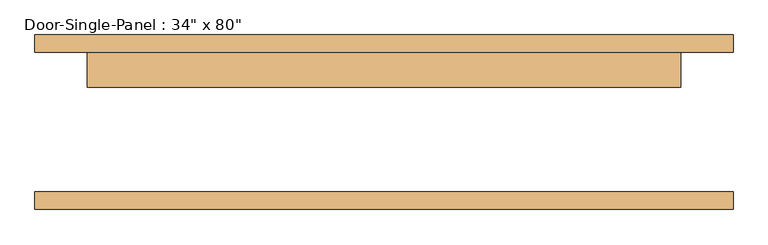
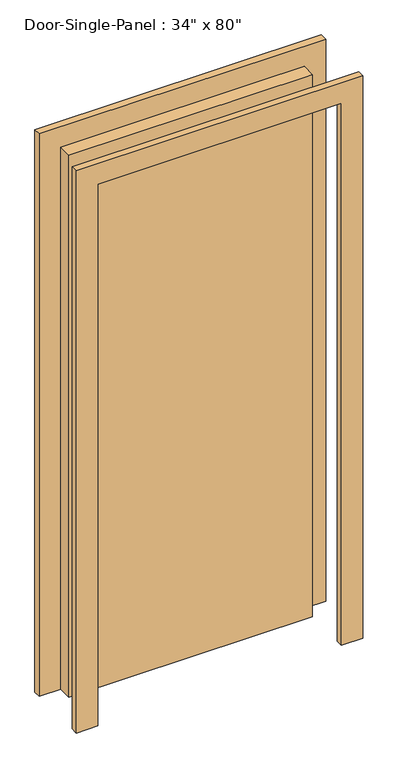
"""IFC4 building model written with IfcOpenShell, lengths in millimetres: door geometry."""

from ifc_helpers import new_model, si_unit, frame, origin, origin_with_axes, place, context, project, spatial, polyline, outline, extrude, source, transform, mapped, element, save


def door_10fd3a06(model_context):
    return source(origin(), model_context, "Body", "SweptSolid", [
        extrude(outline(polyline([(431.8, 50.8), (-431.8, 50.8), (-431.8, 101.6), (431.8, 101.6), (431.8, 50.8)])), origin_with_axes(), (0.0, 0.0, 1.0), 2032.0),
        extrude(outline(polyline([(2108.2, -508.0), (0.0, -508.0), (0.0, -431.8), (2032.0, -431.8), (2032.0, 431.8), (0.0, 431.8), (0.0, 508.0), (2108.2, 508.0), (2108.2, -508.0)])), frame((0.0, 101.6, 0.0), z_axis=(0.0, 1.0, 0.0), x_axis=(0.0, 0.0, 1.0)), (0.0, 0.0, 1.0), 25.4),
        extrude(outline(polyline([(2108.2, 508.0), (2108.2, -508.0), (0.0, -508.0), (0.0, -431.8), (2032.0, -431.8), (2032.0, 431.8), (0.0, 431.8), (0.0, 508.0), (2108.2, 508.0)])), frame((0.0, -127.0, 0.0), z_axis=(0.0, 1.0, 0.0), x_axis=(0.0, 0.0, 1.0)), (0.0, 0.0, 1.0), 25.4),
    ])


if __name__ == "__main__":
    model = new_model("IFC4")
    model_context = context("Model", 3, world=origin())
    ifc_project = project(units=[si_unit("LENGTHUNIT", "METRE", prefix="MILLI")], contexts=[model_context])
    site = spatial("IfcSite", under=ifc_project)
    building = spatial("IfcBuilding", under=site)
    placement = place(None, origin())
    door_shape = door_10fd3a06(model_context)
    element("IfcDoor", 1, ObjectType="Door-Single-Panel : 34\" x 80\"", at=placement, inside=building, context=model_context, shape_type="MappedRepresentation", body=[
        mapped(door_shape, transform((0.0, 0.0, 0.0), x_axis=(1.0, 0.0, 0.0), y_axis=(0.0, 1.0, 0.0), z_axis=(0.0, 0.0, 1.0))),
    ])
    save(model, "model.ifc")

# Revit data of these elements
# Type "Door-Single-Panel : 34\" x 80\""
#   Type Mark = "9"
#   Construction Type Id = "DOOR"
#   Assembly Code = "C1020300"
#   Analytic Construction = "Wooden"
#   Thickness = 0' - 2"
#   Thermal Resistance (R) = 2.5876 (h·ft²·°F)/BTU
#   Swing Angle [instance default] = 90.00°
#   Heat Transfer Coefficient (U) = 0.3865 BTU/(h·ft²·°F)
#   Height = 6' - 8"
#   Trim Projection Ext = 0' - 1"
#   Trim Projection Int = 0' - 1"
#   Trim Width = 0' - 3"
#   Width = 2' - 10"
#   Define Thermal Properties by = 1
#   Panel Material = Wood - Birch - Solid Stained Light Low Gloss
#   Trim Material = Paint - Sienna
#   Visual Light Transmittance = 0
#   Solar Heat Gain Coefficient = 0
#   Function = (empty or 0)
#   Wall Closure = (empty or 0)
# Element 1 (IfcDoor, "Door-Single-Panel : 34\" x 80\"")
#   Materials on its faces: "Paint - Sienna", "Wood - Birch - Solid Stained Light Low Gloss"
# Materials
#   "Wood - Birch - Solid Stained Light Low Gloss": class "Wood", colour RGB 210 159 95, transparency 0, Cost = 0
#   "Paint - Sienna": colour RGB 118 70 51, transparency 0, Cost = 0
